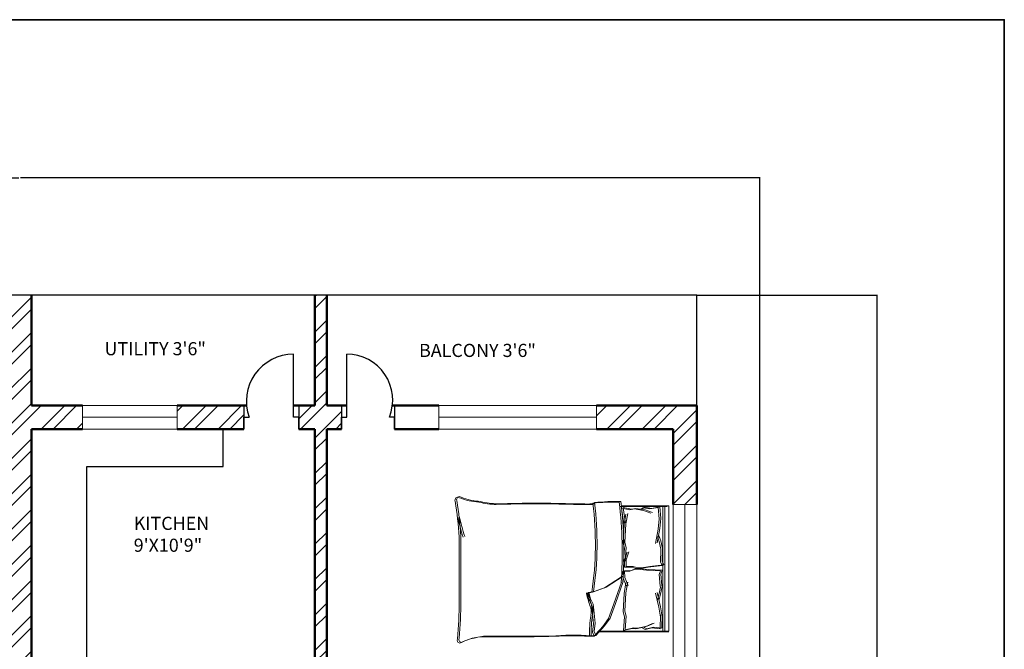
# Model space of a CAD drawing. Units: inches. Extents: x 1980 to 2738, y 1471 to 2568.
# Tile 22 of 22: x 2363 to 2738, y 2328 to 2568. Entities that reach past the tile are written whole.
import ezdxf

# ---------------------------------------------------------------- set-up
doc = ezdxf.new("R2010")
doc.units = ezdxf.units.IN
for name, color, linetype, lineweight in [('A-ANNO-DIMS', 2, 'Continuous', 18), ('A-ANNO-TTLB', 7, 'Continuous', 35), ('A-AREA-IDEN', 7, 'Continuous', 18), ('A-DOOR', 31, 'Continuous', 25), ('A-FLOR-BALC', 7, 'Continuous', 25), ('A-FLOR-CASE', 8, 'Continuous', 25), ('A-FURN', 8, 'Continuous', 18), ('A-GLAZ', 141, 'Continuous', 18), ('A-WALL', 7, 'Continuous', 50)]:
    doc.layers.add(name, color=color, linetype=linetype, lineweight=lineweight)
doc.layers.add('A-WALL-PATT', color=9, linetype='Continuous', lineweight=13, true_color=0xd19cc7)
doc.styles.get("Standard").update_dxf_attribs({"font": 'arial.ttf'})
doc.dimstyles.get("Standard").update_dxf_attribs({"dimtxt": 0.18, "dimasz": 0.18, "dimexe": 0.18, "dimexo": 0.0625, "dimgap": 0.09, "dimtad": 0, "dimtih": 1, "dimtoh": 1, "dimdec": 4, "dimzin": 0, "dimdsep": 46, "dimtxsty": 'Standard', "dimcen": 0.09, "dimadec": 0, "dimazin": 0, "dimtfac": 1, "dimtdec": 4, "dimtofl": 0, "dimtmove": 0, "dimatfit": 3, "dimfxl": 1, "dimtolj": 1, "dimtzin": 0, "dimarcsym": 0})

# ---------------------------------------------------------------- blocks, each defined once
blk = doc.blocks.new('BED-DOUBLE')
for p, q in [((27.75, 52.87), (24.5, 49.16)), ((27.75, 52.87), (24.5, 49.16)), ((28.38, 53.1), (25.13, 49.39)), ((28.38, 53.1), (25.13, 49.39)), ((29.49, 52.95), (27.75, 52.87, 3.87)), ((29.49, 52.95), (27.75, 52.87, 3.87)), ((28.36, 51.33), (27.75, 52.87)), ((28.36, 51.33), (27.75, 52.87)), ((30.13, 53.18), (28.38, 53.1, 3.87)), ((30.13, 53.18), (28.38, 53.1, 3.87)), ((29, 51.56), (28.38, 53.1)), ((29, 51.56), (28.38, 53.1)), ((0, 51.49), (0.64, 51.49)), ((0, 51.27), (26.61, 51.27)), ((0, 51.27), (26.61, 51.27)), ((0, 51.27), (0, 3.48)), ((0.64, 51.49), (27.25, 51.49)), ((0.64, 51.49), (27.25, 51.49)), ((1.53, 3.48), (1.53, 51.27)), ((1.53, 3.48), (1.53, 51.27)), ((2.17, 3.7), (2.17, 51.49)), ((2.17, 3.7), (2.17, 51.49)), ((2.56, 50.11), (2.46, 44.71)), ((2.56, 50.11), (2.46, 44.71)), ((2.56, 50.11), (5.77, 49.73)), ((2.56, 50.11), (5.77, 49.73)), ((3.2, 50.34), (3.1, 44.94)), ((3.2, 50.34), (3.1, 44.94)), ((3.2, 50.34), (6.41, 49.96)), ((3.2, 50.34), (6.41, 49.96)), ((8.26, 49.31), (5.58, 48.13)), ((8.26, 49.31), (5.58, 48.13)), ((5.77, 49.73), (8.34, 50.33)), ((5.77, 49.73), (8.34, 50.33)), ((8.9, 49.54), (6.22, 48.36)), ((8.9, 49.54), (6.22, 48.36)), ((6.41, 49.96), (8.98, 50.56)), ((6.41, 49.96), (8.98, 50.56)), ((11.83, 50.11), (8.26, 49.31)), ((11.83, 50.11), (8.26, 49.31)), ((8.34, 50.33), (9.38, 49.81)), ((8.34, 50.33), (9.38, 49.81)), ((12.47, 50.34), (8.9, 49.54)), ((12.47, 50.34), (8.9, 49.54)), ((8.98, 50.56), (10.02, 50.04)), ((8.98, 50.56), (10.02, 50.04)), ((13.43, 49.92), (11.83, 50.11)), ((13.43, 49.92), (11.83, 50.11)), ((14.07, 50.15), (12.47, 50.34)), ((14.07, 50.15), (12.47, 50.34)), ((16.57, 50.7), (13.43, 49.92)), ((16.57, 50.7), (13.43, 49.92)), ((17.21, 50.93), (14.07, 50.15)), ((17.21, 50.93), (14.07, 50.15)), ((16.17, 45.57), (16.57, 50.7)), ((16.17, 45.57), (16.57, 50.7)), ((16.81, 45.8), (17.21, 50.93)), ((16.81, 45.79), (17.21, 50.93)), ((24.5, 49.16), (22.33, 46.22)), ((24.5, 49.16), (22.33, 46.22)), ((25.13, 49.39), (22.97, 46.45)), ((25.13, 49.39), (22.97, 46.45)), ((28.06, 48.23), (28.36, 51.33)), ((28.06, 48.23), (28.36, 51.33)), ((28.69, 48.46), (29, 51.56)), ((28.69, 48.46), (29, 51.56)), ((2.46, 44.71), (2.54, 45.71)), ((2.46, 44.71), (2.54, 45.71)), ((2.54, 45.71), (3.07, 41.91)), ((2.54, 45.71), (3.07, 41.91)), ((3.1, 44.94), (3.18, 45.94)), ((3.1, 44.94), (3.18, 45.94)), ((3.18, 45.94), (3.71, 42.14)), ((3.18, 45.94), (3.71, 42.14)), ((16.73, 43.61), (16.17, 45.57)), ((16.73, 43.61), (16.17, 45.57)), ((17.37, 43.83), (16.81, 45.8)), ((17.37, 43.83), (16.81, 45.79)), ((22.33, 46.22), (20.32, 40.64)), ((22.33, 46.22), (20.32, 40.64)), ((22.97, 46.45), (20.96, 40.87)), ((22.97, 46.45), (20.96, 40.87)), ((28.36, 44.36), (28.06, 48.23)), ((28.36, 44.36), (28.06, 48.23)), ((29, 44.59), (28.69, 48.46)), ((29, 44.59), (28.69, 48.46)), ((3.07, 41.91), (4.42, 36.5)), ((3.07, 41.91), (4.42, 36.5)), ((3.71, 42.14), (5.06, 36.72)), ((3.71, 42.14), (5.06, 36.72)), ((16.29, 36.6), (16.73, 43.61)), ((16.29, 36.6), (16.73, 43.61)), ((16.93, 36.82), (17.37, 43.83)), ((16.93, 36.82), (17.37, 43.83)), ((28.83, 40.95), (28.36, 44.36)), ((28.83, 40.95), (28.36, 44.36)), ((29.47, 41.18), (29, 44.59)), ((29.47, 41.18), (29, 44.59)), ((3.67, 39.2), (3.08, 37.14)), ((3.67, 39.2), (3.08, 37.14)), ((4.31, 39.43), (3.72, 37.36)), ((4.31, 39.43), (3.72, 37.36)), ((20.32, 40.64), (17.38, 32.31)), ((20.32, 40.64), (17.38, 32.31)), ((20.96, 40.87), (18.02, 32.53)), ((20.96, 40.87), (18.02, 32.53)), ((29.76, 38.94), (28.83, 40.95)), ((29.76, 38.94), (28.83, 40.95)), ((30.4, 39.17), (29.47, 41.18)), ((30.4, 39.17), (29.47, 41.18)), ((30.38, 36.46), (29.76, 38.94)), ((30.38, 36.46), (29.76, 38.94)), ((31.02, 36.69), (30.4, 39.17)), ((31.02, 36.69), (30.4, 39.17)), ((79.24, 15.06), (79.24, 39.68)), ((79.24, 15.06), (79.24, 39.68)), ((79.88, 15.29), (79.88, 39.91)), ((79.88, 15.29), (79.88, 39.91)), ((3.08, 37.14), (2.54, 34.2)), ((3.08, 37.14), (2.54, 34.2)), ((2.54, 34.2), (2.56, 33.88)), ((2.54, 34.2), (2.56, 33.88)), ((2.56, 33.88), (2.98, 29.46)), ((2.56, 33.88), (2.98, 29.46)), ((3.72, 37.36), (3.18, 34.43)), ((3.72, 37.36), (3.18, 34.43)), ((3.18, 34.43), (3.2, 34.11)), ((3.18, 34.43), (3.2, 34.11)), ((3.2, 34.11), (3.62, 29.68)), ((3.2, 34.11), (3.62, 29.68)), ((16.74, 30.75), (15.45, 33.82)), ((16.74, 30.75), (15.45, 33.82)), ((15.63, 32.56), (16.29, 36.6)), ((15.63, 32.56), (16.29, 36.6)), ((17.38, 30.98), (16.09, 34.05)), ((17.38, 30.98), (16.09, 34.05)), ((16.27, 32.79), (16.93, 36.82)), ((16.27, 32.79), (16.93, 36.82)), ((17.38, 30.26), (23.88, 34.45)), ((17.38, 30.26), (23.88, 34.45)), ((18.02, 30.49), (24.52, 34.68)), ((18.02, 30.49), (24.52, 34.68)), ((23.88, 34.45), (28.36, 36.15)), ((23.88, 34.45), (28.36, 36.15)), ((24.52, 34.68), (29, 36.38)), ((24.52, 34.68), (29, 36.38)), ((28.36, 36.15), (30.38, 36.46)), ((28.36, 36.15), (30.38, 36.46)), ((29, 36.38), (31.02, 36.69)), ((29, 36.38), (31.02, 36.69)), ((16.89, 28.3), (16.74, 30.75)), ((16.89, 28.3), (16.74, 30.75)), ((17.53, 28.53), (17.38, 30.98)), ((17.53, 28.53), (17.38, 30.98)), ((1.87, 25.98), (7.22, 26.56)), ((1.87, 25.98), (7.22, 26.56)), ((2.98, 29.46), (2.49, 27.98)), ((2.98, 29.46), (2.49, 27.98)), ((2.49, 27.98), (7.87, 27.73)), ((2.49, 27.98), (7.87, 27.73)), ((2.51, 26.21), (7.86, 26.79)), ((2.51, 26.21), (7.86, 26.79)), ((3.62, 29.68), (3.13, 28.21)), ((3.62, 29.68), (3.13, 28.21)), ((3.13, 28.21), (8.51, 27.96)), ((3.13, 28.21), (8.51, 27.96)), ((7.22, 26.56), (10.4, 27.14)), ((7.22, 26.56), (10.4, 27.14)), ((7.86, 26.79), (11.04, 27.37)), ((7.86, 26.79), (11.04, 27.37)), ((7.87, 27.73), (11.08, 27.36)), ((7.87, 27.73), (11.08, 27.35)), ((8.51, 27.96), (11.72, 27.58)), ((8.51, 27.96), (11.72, 27.58)), ((10.4, 27.14), (11.7, 27.14)), ((10.4, 27.14), (11.7, 27.14)), ((11.04, 27.37), (12.34, 27.37)), ((11.04, 27.37), (12.34, 27.37)), ((11.08, 27.36), (12.38, 27.44)), ((11.08, 27.35), (12.38, 27.44)), ((11.7, 27.14), (13.58, 26.56)), ((11.7, 27.14), (13.58, 26.56)), ((11.72, 27.58), (13.02, 27.66)), ((11.72, 27.58), (13.02, 27.66)), ((12.34, 27.37), (14.22, 26.79)), ((12.34, 27.37), (14.22, 26.79)), ((12.38, 27.44), (14.22, 28.13)), ((12.38, 27.44), (14.22, 28.13)), ((13.02, 27.66), (14.86, 28.36)), ((13.02, 27.66), (14.86, 28.36)), ((13.58, 26.56), (16.26, 26.56)), ((13.58, 26.56), (16.26, 26.56)), ((14.22, 28.13), (16.89, 28.3)), ((14.22, 28.13), (16.89, 28.3)), ((14.22, 26.79), (16.9, 26.79)), ((14.22, 26.79), (16.9, 26.79)), ((14.86, 28.36), (17.53, 28.53)), ((14.86, 28.36), (17.53, 28.53)), ((16.26, 26.56), (16.26, 24.1)), ((16.26, 26.56), (16.26, 24.1)), ((16.9, 26.79), (16.9, 24.33)), ((16.9, 26.79), (16.9, 24.33)), ((2.45, 24.54), (1.87, 25.98)), ((2.45, 24.54), (1.87, 25.98)), ((2.3, 20.09), (2.45, 24.54)), ((2.3, 20.09), (2.45, 24.54)), ((3.09, 24.77), (2.51, 26.21)), ((3.09, 24.77), (2.51, 26.21)), ((2.94, 20.32), (3.09, 24.77)), ((2.94, 20.32), (3.09, 24.77)), ((16.26, 24.1), (15.17, 20.96)), ((16.26, 24.1), (15.17, 20.96)), ((16.9, 24.33), (15.81, 21.19)), ((16.9, 24.33), (15.81, 21.19)), ((16.17, 19.38), (16.57, 24.52)), ((16.17, 19.38), (16.57, 24.52)), ((16.81, 19.61), (17.21, 24.74)), ((16.81, 19.61), (17.21, 24.74)), ((2.3, 19.77), (2.3, 20.09)), ((2.3, 19.77), (2.3, 20.09)), ((3.03, 16.88), (2.3, 19.77)), ((3.03, 16.88), (2.3, 19.77)), ((2.94, 20), (2.94, 20.32)), ((2.94, 20), (2.94, 20.32)), ((3.67, 17.11), (2.94, 20)), ((3.67, 17.11), (2.94, 20)), ((16.73, 17.42), (16.17, 19.38)), ((16.73, 17.42), (16.17, 19.38)), ((17.37, 17.65), (16.81, 19.61)), ((17.37, 17.65), (16.81, 19.61)), ((3.75, 14.86), (3.03, 16.88)), ((3.75, 14.85), (3.03, 16.88)), ((3.32, 12.11), (4.33, 17.6)), ((3.32, 12.11), (4.33, 17.6)), ((4.39, 15.08), (3.67, 17.11)), ((4.39, 15.08), (3.67, 17.11)), ((3.96, 12.34), (4.97, 17.83)), ((3.96, 12.34), (4.97, 17.83)), ((16.29, 10.41), (16.73, 17.42)), ((16.29, 10.41), (16.73, 17.42)), ((16.93, 10.64), (17.37, 17.65)), ((16.93, 10.64), (17.37, 17.65)), ((3.03, 8.29), (3.32, 12.11)), ((3.03, 8.28), (3.32, 12.11)), ((3.67, 8.51), (3.96, 12.34)), ((3.67, 8.51), (3.96, 12.34)), ((3.01, 8.18), (3.03, 8.29)), ((3.01, 8.18), (3.03, 8.28)), ((3.34, 3.9), (3.01, 8.18)), ((3.34, 3.9), (3.01, 8.18)), ((3.65, 8.41), (3.67, 8.51)), ((3.65, 8.41), (3.67, 8.51)), ((3.98, 4.13), (3.65, 8.41)), ((3.98, 4.13), (3.65, 8.41)), ((15.63, 6.38), (16.29, 10.41)), ((15.63, 6.38), (16.29, 10.41)), ((16.27, 6.61), (16.93, 10.64)), ((16.27, 6.61), (16.93, 10.64)), ((16.29, 10.41), (16.62, 9.28)), ((16.29, 10.41), (16.62, 9.28)), ((16.62, 9.28), (17.34, 4.18)), ((16.62, 9.28), (17.34, 4.18)), ((16.93, 10.64), (17.26, 9.51)), ((16.93, 10.64), (17.26, 9.51)), ((17.26, 9.51), (17.98, 4.41)), ((17.26, 9.51), (17.98, 4.41)), ((3.32, 3.89), (6.5, 4.47)), ((3.32, 3.89), (6.5, 4.47)), ((3.96, 4.12), (7.14, 4.7)), ((3.96, 4.12), (7.14, 4.7)), ((8.95, 5.05), (6.21, 6.06)), ((8.95, 5.05), (6.21, 6.06)), ((6.5, 4.47), (9.1, 4.04)), ((6.5, 4.47), (9.1, 4.04)), ((9.59, 5.28), (6.85, 6.29)), ((9.59, 5.28), (6.85, 6.29)), ((7.14, 4.7), (9.74, 4.27)), ((7.14, 4.7), (9.74, 4.27)), ((12.57, 4.47), (8.95, 5.05)), ((12.57, 4.47), (8.95, 5.05)), ((9.1, 4.04), (10.11, 4.62)), ((9.1, 4.04), (10.11, 4.62)), ((13.21, 4.7), (9.59, 5.28)), ((13.21, 4.7), (9.59, 5.28)), ((9.74, 4.27), (10.75, 4.85)), ((9.74, 4.27), (10.75, 4.85)), ((14.16, 4.76), (12.57, 4.47)), ((14.16, 4.76), (12.57, 4.47)), ((14.8, 4.99), (13.21, 4.7)), ((14.8, 4.99), (13.21, 4.7)), ((17.34, 4.18), (14.16, 4.76)), ((17.34, 4.18), (14.16, 4.76)), ((17.98, 4.41), (14.8, 4.99)), ((17.98, 4.41), (14.8, 4.99)), ((18.11, 3.48), (0, 3.48)), ((18.11, 3.48), (0, 3.48)), ((18.75, 3.7), (0.64, 3.7)), ((18.75, 3.7), (0.64, 3.7))]:
    blk.add_line(p, q)
for centre, radius, start, end in [((-6.66, 51.33), 36.18, 349.8763, 2.5657), ((-6.66, 51.33), 36.18, 349.8763, 2.5657), ((36.31, 182.27), 129.5, 266.9791, 273.8365), ((36.31, 182.27), 129.5, 266.9791, 273.8365), ((-6.02, 51.56), 36.18, 349.8763, 2.5657), ((-6.02, 51.56), 36.18, 349.8763, 2.5657), ((36.95, 182.49), 129.5, 266.9791, 273.8365), ((36.95, 182.49), 129.5, 266.9791, 273.8365), ((67.82, -4508.74), 4561.86, 90.00217, 90.28689), ((67.82, -4508.74), 4561.86, 90.00217, 90.28689), ((68.46, -4508.51), 4561.86, 90.00217, 90.28689), ((68.46, -4508.52), 4561.86, 90.00217, 90.28689), ((68.67, 76.16), 23.07, 267.4714, 296.4681), ((68.67, 76.16), 23.07, 267.4714, 296.4681), ((69.31, 76.39), 23.07, 267.4714, 296.4681), ((69.31, 76.39), 23.07, 267.4714, 296.4681), ((78.87, 54.41), 1.1, 332.6588, 86.02), ((78.87, 54.41), 1.1, 332.6588, 86.02), ((212.28, 41.15), 133.04, 174.4998, 180.6351), ((212.28, 41.15), 133.04, 174.4998, 180.6351), ((79.51, 54.64), 1.1, 332.6588, 86.02), ((79.51, 54.64), 1.1, 332.6588, 86.02), ((212.92, 41.38), 133.04, 174.4998, 180.6351), ((212.92, 41.38), 133.04, 174.4998, 180.6351), ((35.71, 43.97), 6.22, 168.6608, 203.7384), ((35.71, 43.97), 6.22, 168.6608, 203.7384), ((35.07, 43.74), 6.22, 168.6608, 203.7384), ((35.07, 43.74), 6.22, 168.6608, 203.7384), ((2.12, 31.38), 29.65, 10.6617, 19.8806), ((2.12, 31.38), 29.65, 10.6617, 19.8806), ((1.48, 31.15), 29.65, 10.6617, 19.8806), ((1.48, 31.15), 29.65, 10.6617, 19.8806), ((156.32, 17.76), 129.02, 171.7845, 186.9006), ((156.32, 17.76), 129.02, 171.7845, 186.9006), ((156.96, 17.98), 129.02, 171.7845, 186.9006), ((156.96, 17.98), 129.02, 171.7845, 186.9006), ((30.44, 36.64), 0.185, 250.2464, 1.1377), ((30.44, 36.64), 0.185, 250.2464, 1.1377), ((31.08, 36.86), 0.185, 250.2464, 1.1377), ((31.08, 36.86), 0.185, 250.2464, 1.1377), ((182.05, 21.36), 164.97, 176.0865, 186.7821), ((182.05, 21.36), 164.97, 176.0865, 186.7821), ((182.69, 21.59), 164.97, 176.0865, 186.7821), ((182.69, 21.59), 164.97, 176.0865, 186.7821), ((-23.71, -17.22), 106.46, 13.3832, 17.7053), ((-23.71, -17.22), 106.46, 13.3832, 17.7053), ((-23.07, -16.99), 106.46, 13.3832, 17.7053), ((-23.07, -16.99), 106.46, 13.3832, 17.7053), ((200.84, 21.43), 121.76, 182.9958, 189.4091), ((200.84, 21.43), 121.76, 182.9958, 189.4091), ((201.48, 21.66), 121.76, 182.9958, 189.4091), ((201.48, 21.66), 121.76, 182.9958, 189.4091), ((20.1, 85.16), 83.31, 268.7218, 275.604), ((20.1, 85.16), 83.31, 268.7218, 275.604), ((20.74, 85.39), 83.31, 268.7218, 275.604), ((20.74, 85.39), 83.31, 268.7218, 275.604), ((31.17, -167.31), 170.11, 88.4762, 91.0082), ((31.17, -167.31), 170.11, 88.4762, 91.0082), ((31.81, -167.08), 170.11, 88.4762, 91.0082), ((31.81, -167.08), 170.11, 88.4762, 91.0082), ((50.61, 484.82), 482.31, 268.2277, 271.7185), ((50.61, 484.82), 482.31, 268.2277, 271.7185), ((51.25, 485.05), 482.31, 268.2277, 271.7185), ((51.25, 485.05), 482.31, 268.2277, 271.7185), ((64.51, -26.9), 29.63, 76.0648, 88.9113), ((64.51, -26.9), 29.63, 76.0648, 88.9113), ((65.15, -26.67), 29.63, 76.0648, 88.9113), ((65.15, -26.67), 29.63, 76.0648, 88.9113), ((70.28, -21.66), 23.56, 67.9751, 86.652), ((70.28, -21.66), 23.56, 67.9751, 86.652), ((70.91, -21.43), 23.56, 67.9751, 86.652), ((70.91, -21.43), 23.56, 67.9751, 86.652), ((79.72, 1.09), 1.09, 236.1736, 23.4781), ((79.72, 1.09), 1.09, 236.1736, 23.4781), ((80.36, 1.32), 1.09, 236.1736, 23.4781), ((80.36, 1.32), 1.09, 236.1736, 23.4781)]:
    blk.add_arc(centre, radius, start, end)
blk = doc.blocks.new('WIN-60IN-WALL')
for p, q in [((0, 9), (0, 0)), ((60, 9), (0, 9)), ((60, 4.5), (60, 9)), ((60, 9), (60, 0)), ((0, 0), (0, 4.5)), ((0, 4.5), (60, 4.5)), ((0, 0), (60, 0))]:
    blk.add_line(p, q)
blk = doc.blocks.new('WIN-36IN-WALL')
for p, q in [((0, 9), (0, 0)), ((0, 9), (36, 9)), ((36, 4.5), (36, 9)), ((36, 9), (36, 0)), ((0, 0), (0, 4.5)), ((0, 4.5), (36, 4.5)), ((36, 0), (0, 0))]:
    blk.add_line(p, q)
blk = doc.blocks.new('*D35')
at = {"layer": 'A-ANNO-DIMS', "color": 0, "lineweight": -2, "transparency": 16777216}
for p, q in [((2081.08, 2291.77), (2081.08, 2507.54)), ((2081.26, 2507.36), (2362.79, 2507.36)), ((2644.9, 2507.36), (2363.37, 2507.36)), ((2645.08, 2291.77), (2645.08, 2507.54))]:
    blk.add_line(p, q, dxfattribs=at)
at = {"layer": 'A-ANNO-DIMS', "color": 0, "transparency": 16777216}
for points in [[(2081.26, 2507.39), (2081.26, 2507.33), (2081.08, 2507.36)], [(2644.9, 2507.39), (2644.9, 2507.33), (2645.08, 2507.36)]]:
    blk.add_solid(points, dxfattribs=at)
at = {"layer": 'Defpoints', "color": 0, "transparency": 16777216}
for p in [(2645.08, 2507.36), (2081.08, 2291.71), (2645.08, 2291.71)]:
    blk.add_point(p, dxfattribs=at)
at = {"layer": 'A-ANNO-DIMS', "color": 0, "transparency": 16777216, "insert": (2363.08, 2507.36), "char_height": 0.18, "attachment_point": 5}
blk.add_mtext('\\A1;564', dxfattribs=at)
blk = doc.blocks.new('*D39')
at = {"layer": 'A-ANNO-DIMS', "color": 0, "lineweight": -2, "transparency": 16777216}
for p, q in [((2621.15, 2462.71), (2689.91, 2462.71)), ((2689.73, 2462.53), (2689.73, 2279.14)), ((2689.73, 2095.39), (2689.73, 2278.77)), ((2579.97, 2095.21), (2689.91, 2095.21))]:
    blk.add_line(p, q, dxfattribs=at)
at = {"layer": 'A-ANNO-DIMS', "color": 0, "transparency": 16777216}
for points in [[(2689.7, 2462.53), (2689.76, 2462.53), (2689.73, 2462.71)], [(2689.7, 2095.39), (2689.76, 2095.39), (2689.73, 2095.21)]]:
    blk.add_solid(points, dxfattribs=at)
at = {"layer": 'Defpoints', "color": 0, "transparency": 16777216}
for p in [(2621.08, 2462.71), (2689.73, 2462.71), (2579.9, 2095.21)]:
    blk.add_point(p, dxfattribs=at)
at = {"layer": 'A-ANNO-DIMS', "color": 0, "transparency": 16777216, "insert": (2689.73, 2278.96), "char_height": 0.18, "attachment_point": 5}
blk.add_mtext('\\A1;367.5', dxfattribs=at)

msp = doc.modelspace()

# ---------------------------------------------------------------- hatches: boundary and pattern name
at = {"layer": 'A-WALL-PATT'}
h = msp.add_hatch(dxfattribs=at)
h.set_pattern_fill('ANSI32', color=256)
h.paths.add_polyline_path([(2257.5661, 2416.2064), (2257.5661, 2420.7064), (2250.5833, 2420.7064), (2250.5833, 2462.7064), (2246.0833, 2462.7064), (2246.0833, 2420.7064), (2237.0791, 2420.7064), (2237.0791, 2411.7064), (2246.0833, 2411.7064), (2246.0833, 2291.7064), (2242.6109, 2291.7064), (2242.6109, 2287.2064), (2246.0833, 2287.2064), (2250.5833, 2287.2064), (2250.5833, 2291.7064), (2250.5833, 2411.7064), (2257.5661, 2411.7064)])
h.paths.add_polyline_path([(2387.0396, 2416.2064), (2387.0396, 2420.7064), (2367.5833, 2420.7064), (2367.5833, 2462.7064), (2358.5833, 2462.7064), (2358.5833, 2420.7064), (2329.3087, 2420.7064), (2329.3087, 2411.7064), (2358.5833, 2411.7064), (2358.5833, 2321.7275), (2358.5833, 2309.7064), (2347.3089, 2309.7064), (2293.3089, 2309.7064), (2293.3089, 2259.0771), (2297.8089, 2259.0771), (2297.8089, 2305.2064), (2347.3089, 2305.2064), (2347.3089, 2284.7412), (2351.8089, 2284.7412), (2351.8089, 2305.2064), (2372.3188, 2305.2064), (2372.3761, 2284.3899), (2377.0295, 2284.3899), (2377.0295, 2299.3058), (2377.0295, 2305.2064), (2426.5295, 2305.2064), (2426.5295, 2257.5573), (2431.0295, 2257.5573), (2431.0295, 2309.7064), (2377.0295, 2309.7064), (2367.5833, 2309.7064), (2367.5833, 2321.7275), (2367.5833, 2411.7064), (2387.0396, 2411.7064)])
h.paths.add_polyline_path([(2448.5267, 2416.2064), (2448.5267, 2420.7064), (2423.0396, 2420.7064), (2423.0396, 2411.7064), (2448.5267, 2411.7064)])
h.paths.add_polyline_path([(2130.9128, 2416.2064), (2130.9128, 2420.7064), (2105.0833, 2420.7064), (2105.0833, 2386.6942), (2114.0833, 2386.6942), (2114.0833, 2411.7064), (2130.9128, 2411.7064)])
h.paths.add_polyline_path([(2212.9478, 2420.7064), (2190.9128, 2420.7064), (2190.9128, 2411.7064), (2212.9478, 2411.7064), (2212.9478, 2416.2064)])
h.paths.add_polyline_path([(2114.0833, 2326.6942), (2105.0833, 2326.6942), (2105.0833, 2291.7064), (2081.0833, 2291.7064), (2081.0833, 2287.2064), (2105.0833, 2287.2064), (2105.0833, 2276.1935), (2114.0833, 2276.1935), (2114.0833, 2287.2064), (2166.3825, 2287.2064), (2166.3825, 2289.4564), (2166.3825, 2291.7064), (2114.0833, 2291.7064)])
h.paths.add_polyline_path([(2114.0833, 2252.1935), (2105.0833, 2252.1935), (2105.0833, 2233.2064), (2081.0833, 2233.2064), (2081.0833, 2228.7064), (2105.0833, 2228.7064), (2105.0833, 2213.4478), (2114.0833, 2213.4478), (2114.0833, 2228.7064), (2195.0833, 2228.7064), (2199.5833, 2228.7064), (2208.4455, 2228.7064), (2208.4455, 2230.9564), (2208.4455, 2233.2064), (2199.5833, 2233.2064), (2199.5833, 2287.2064), (2206.8904, 2287.2064), (2206.8904, 2289.4564), (2206.8904, 2291.7064), (2189.446, 2291.7064), (2189.446, 2289.4564), (2189.446, 2287.2064), (2195.0833, 2287.2064), (2195.0833, 2233.2064), (2114.0833, 2233.2064)])
h.paths.add_polyline_path([(2114.0833, 2153.4478), (2109.5833, 2153.4478), (2105.0833, 2153.4478), (2105.0833, 2135.2374), (2114.0833, 2135.2374)], flags=17)
h.paths.add_polyline_path([(2135.9619, 2095.4081), (2140.1805, 2095.4081), (2140.1805, 2104.2064), (2114.0833, 2104.2064), (2114.0833, 2110.3997), (2109.5833, 2110.3997), (2105.0833, 2110.3997), (2105.0833, 2104.2064), (2081.0833, 2104.2064), (2081.0833, 2099.7064), (2105.0833, 2099.7064), (2127.5416, 2099.8532), (2127.5416, 2056.9393), (2136.2133, 2056.9393)], flags=17)
h.paths.add_polyline_path([(2255.4895, 2104.2064), (2250.5833, 2104.2064), (2250.5833, 2233.2064), (2246.0833, 2233.2064), (2242.4941, 2233.2064), (2242.4941, 2228.7064), (2246.0833, 2228.7064), (2246.0833, 2104.2064), (2163.6825, 2104.2064), (2163.6825, 2099.8072), (2163.6825, 2095.4081), (2191.4325, 2095.4081), (2191.4325, 2011.2064), (2186.0833, 2011.2064), (2136.5143, 2010.8824), (2136.3702, 2032.9403), (2131.9559, 2032.9115), (2127.5416, 2032.8826), (2127.5416, 2006.7064), (2105.0833, 2006.7064), (2081.0833, 2006.7064), (2081.0833, 2002.2064), (2105.0833, 2002.2064), (2105.0833, 1995.9329), (2114.0833, 1995.9329), (2114.0833, 2002.2064), (2246.0833, 2002.2064), (2246.0833, 1877.7064), (2242.1358, 1877.7064), (2242.1358, 1873.2064), (2250.5833, 1873.2064), (2250.5833, 2002.2064), (2255.3335, 2002.2064), (2255.3335, 2011.2064), (2195.9325, 2011.2064), (2195.9325, 2095.2064), (2255.4895, 2095.2064), (2255.4895, 2099.5471)])
h.paths.add_polyline_path([(2199.5833, 1873.2064), (2209.827, 1873.2064), (2209.827, 1875.4564), (2209.827, 1877.7064), (2114.0833, 1877.7064), (2114.0833, 1890.0968), (2105.0833, 1890.0968), (2105.0833, 1877.7064), (2081.0833, 1877.7064), (2081.0833, 1873.2064), (2105.0833, 1873.2064), (2105.0833, 1857.7279), (2114.0833, 1857.7279), (2114.0833, 1873.2064), (2195.0833, 1873.2064), (2195.0833, 1819.2064), (2190.298, 1819.2064), (2190.298, 1814.7064), (2209.8976, 1814.7064), (2209.8976, 1816.9564), (2209.8976, 1819.2064), (2199.5833, 1819.2064)])
h.paths.add_polyline_path([(2114.0833, 1814.7064), (2166.2538, 1814.7064), (2166.2538, 1816.9564), (2166.2538, 1819.2064), (2114.0833, 1819.2064), (2114.0833, 1833.7279), (2109.5833, 1833.7279), (2105.0833, 1833.7279), (2105.0833, 1819.2064), (2081.0833, 1819.2064), (2081.0833, 1814.7064), (2105.0833, 1814.7064), (2105.0833, 1782.5516), (2114.0833, 1782.5516)])
h.paths.add_polyline_path([(2114.0833, 1722.5516), (2109.5833, 1722.5516), (2105.0833, 1722.5516), (2105.0833, 1685.7064), (2124.5104, 1685.7064), (2124.5104, 1690.2064), (2124.5104, 1694.7064), (2114.0833, 1694.7064)])
h.paths.add_polyline_path([(2218.8787, 1694.7064), (2184.5104, 1694.7064), (2184.5104, 1685.7064), (2218.8787, 1685.7064), (2218.8787, 1690.2064)])
h.paths.add_polyline_path([(2250.5833, 1819.2064), (2242.6431, 1819.2064), (2242.6431, 1816.9564), (2242.6431, 1814.7064), (2246.0833, 1814.7064), (2246.0833, 1694.7064), (2240.4035, 1694.7064), (2240.4035, 1690.2064), (2240.4035, 1685.7064), (2246.0833, 1685.7064), (2246.0833, 1643.7064), (2250.5833, 1643.7064), (2250.5833, 1685.7064), (2255.9859, 1685.7064), (2255.9859, 1690.2064), (2255.9859, 1694.7064), (2250.5833, 1694.7064)])
h.paths.add_polyline_path([(2297.4764, 1694.7064), (2279.3934, 1694.7064), (2279.3934, 1690.2064), (2279.3934, 1685.7064), (2297.4764, 1685.7064), (2297.4764, 1690.2064)])
h.paths.add_polyline_path([(2377.1596, 1694.7064), (2367.5833, 1694.7064), (2367.5833, 1787.7064), (2431.0295, 1787.7064), (2431.0295, 1792.2064), (2431.0295, 1849.4149), (2428.7795, 1849.4149), (2426.5295, 1849.4149), (2426.5295, 1792.2064), (2421.5833, 1792.2064), (2367.5833, 1792.2064), (2297.8089, 1792.2064), (2297.8089, 1850.2946), (2295.5589, 1850.2946), (2293.3089, 1850.2946), (2293.3089, 1792.2064), (2293.3089, 1787.7064), (2297.8089, 1787.7064), (2358.5833, 1787.7064), (2358.5833, 1694.7064), (2333.4764, 1694.7064), (2333.4764, 1685.7064), (2358.5833, 1685.7064), (2358.5833, 1643.7064), (2367.5833, 1643.7064), (2367.5833, 1685.7064), (2377.1596, 1685.7064)])
h.paths.add_polyline_path([(2442.4912, 1694.7064), (2413.1596, 1694.7064), (2413.1596, 1685.7064), (2442.4912, 1685.7064)])
h.paths.add_polyline_path([(2480.0833, 1814.7064), (2483.4816, 1814.7064), (2483.4816, 1817.9384), (2483.4816, 1819.2064), (2475.5833, 1819.2064), (2475.5833, 1694.7064), (2470.7283, 1694.7064), (2470.7283, 1685.7064), (2475.5833, 1685.7064), (2475.5833, 1643.7064), (2480.0833, 1643.7064), (2480.0833, 1685.7064), (2486.3293, 1685.7064), (2486.3293, 1690.2064), (2486.3293, 1694.7064), (2480.0833, 1694.7064)])
h.paths.add_polyline_path([(2621.0833, 1721.7349), (2612.0833, 1721.7349), (2612.0833, 1694.7064), (2586.1453, 1694.7064), (2586.1453, 1685.7064), (2621.0833, 1685.7064)])
h.paths.add_polyline_path([(2526.1453, 1690.2064), (2526.1453, 1694.7064), (2511.584, 1694.7064), (2511.584, 1690.2064), (2511.584, 1685.7064), (2526.1453, 1685.7064)])
h.paths.add_polyline_path([(2645.0833, 1819.2064), (2621.0833, 1819.2064), (2621.0833, 1835.8527), (2616.5833, 1835.8527), (2612.0833, 1835.8527), (2612.0833, 1819.2064), (2560.2541, 1819.2064), (2560.2541, 1814.7064), (2612.0833, 1814.7064), (2612.0833, 1781.7349), (2621.0833, 1781.7349), (2621.0833, 1814.7064), (2645.0833, 1814.7064)])
h.paths.add_polyline_path([(2645.0833, 1877.7064), (2621.0833, 1877.7064), (2621.0833, 1886.4375), (2612.0833, 1886.4375), (2612.0833, 1877.7064), (2517.1032, 1877.7064), (2517.1032, 1875.4564), (2517.1032, 1873.2064), (2526.5833, 1873.2064), (2526.5833, 1819.2064), (2516.6454, 1819.2064), (2516.6454, 1816.9564), (2516.6454, 1814.7064), (2536.4445, 1814.7064), (2536.4445, 1816.9564), (2536.4445, 1819.2064), (2531.0833, 1819.2064), (2531.0833, 1873.2064), (2612.0833, 1873.2064), (2612.0833, 1859.8527), (2621.0833, 1859.8527), (2621.0833, 1873.2064), (2645.0833, 1873.2064)])
h.paths.add_polyline_path([(2645.0833, 2006.7064), (2621.0833, 2006.7064), (2588.5085, 2006.7064), (2588.5085, 2052.9125), (2579.9045, 2052.9125), (2579.9045, 2011.2064), (2519.9045, 2011.2064), (2519.9045, 2095.2064), (2553.1204, 2095.2064), (2553.1204, 2104.2064), (2480.0833, 2104.2064), (2480.0833, 2228.7064), (2484.3832, 2228.7064), (2484.3832, 2230.9564), (2484.3832, 2233.2064), (2475.5833, 2233.2064), (2475.5833, 2104.2064), (2463.1308, 2104.2064), (2463.1308, 2095.2064), (2501.2463, 2095.2064), (2510.9045, 2095.2064), (2515.4045, 2095.2064), (2515.4045, 2011.2064), (2510.9045, 2011.2064), (2501.2463, 2011.2064), (2462.5957, 2011.2064), (2462.5957, 2002.2064), (2475.5833, 2002.2064), (2475.5833, 1873.2064), (2483.6146, 1873.2064), (2483.6146, 1875.4564), (2483.6146, 1877.7064), (2480.0833, 1877.7064), (2480.0833, 2002.2064), (2612.0833, 2002.2064), (2612.0833, 1996.309), (2621.0833, 1996.309), (2621.0833, 2002.2064), (2645.0833, 2002.2064)])
h.paths.add_polyline_path([(2588.5085, 2099.7277), (2621.0833, 2099.7277), (2645.0833, 2099.7064), (2645.0833, 2104.2064), (2621.0833, 2104.2064), (2621.0833, 2109.0038), (2616.5833, 2109.0038), (2612.0833, 2109.0038), (2612.0833, 2104.2064), (2575.0621, 2104.2064), (2575.0621, 2099.7064), (2575.0621, 2095.2064), (2579.9045, 2095.2064), (2579.9045, 2076.9125), (2588.5085, 2076.9125)], flags=17)
h.paths.add_polyline_path([(2367.5833, 2002.2064), (2373.7228, 2002.2064), (2373.7228, 2006.7064), (2373.7228, 2011.2064), (2350.7889, 2011.2064), (2350.7889, 2006.7064), (2350.7889, 2002.2064), (2358.5833, 2002.2064), (2358.5833, 1877.7064), (2293.3089, 1877.7064), (2293.3089, 1870.4987), (2297.8089, 1870.4987), (2297.8089, 1873.2064), (2347.3089, 1873.2064), (2347.3089, 1847.2208), (2351.8089, 1847.2208), (2351.8089, 1873.2064), (2372.5295, 1873.2064), (2372.5295, 1847.8619), (2377.0295, 1847.8619), (2377.0295, 1873.2064), (2426.5295, 1873.2064), (2426.5295, 1868.7339), (2431.0295, 1868.7339), (2431.0295, 1877.7064), (2367.5833, 1877.7064)])
h.paths.add_polyline_path([(2531.0833, 2287.2064), (2534.2285, 2287.2064), (2534.2285, 2291.7064), (2516.7886, 2291.7064), (2516.7886, 2287.2064), (2526.5833, 2287.2064), (2526.5833, 2233.2064), (2517.9112, 2233.2064), (2517.9112, 2230.9564), (2517.9112, 2228.7064), (2526.5833, 2228.7064), (2531.0833, 2228.7064), (2612.0833, 2228.7064), (2612.0833, 2206.8504), (2621.0833, 2206.8504), (2621.0833, 2228.7064), (2645.0833, 2228.7064), (2645.0833, 2233.2064), (2621.0833, 2233.2064), (2621.0833, 2241.8536), (2616.5833, 2241.8536), (2612.0833, 2241.8536), (2612.0833, 2233.2064), (2531.0833, 2233.2064)])
h.paths.add_polyline_path([(2645.0833, 2291.7064), (2621.0833, 2291.7064), (2621.0833, 2323.0138), (2616.5833, 2323.0138), (2612.0833, 2323.0138), (2612.0833, 2291.7064), (2559.6852, 2291.7064), (2559.6852, 2289.4564), (2559.6852, 2287.2064), (2612.0833, 2287.2064), (2612.0833, 2265.8536), (2621.0833, 2265.8536), (2621.0833, 2287.2064), (2645.0833, 2287.2064)])
h.paths.add_polyline_path([(2621.0833, 2420.7064), (2582.8189, 2420.7064), (2582.8189, 2411.7064), (2612.0833, 2411.7064), (2612.0833, 2383.0138), (2621.0833, 2383.0138)])
h.paths.add_polyline_path([(2480.0833, 2411.7064), (2485.7342, 2411.7064), (2485.7342, 2416.2064), (2485.7342, 2420.7064), (2480.0833, 2420.7064), (2480.0833, 2462.7064), (2475.5833, 2462.7064), (2475.5833, 2420.7064), (2469.4083, 2420.7064), (2469.4083, 2411.7064), (2475.5833, 2411.7064), (2475.5833, 2291.7064), (2475.5833, 2287.2064), (2482.9195, 2287.2064), (2482.9195, 2289.4564), (2482.9195, 2291.7064), (2480.0833, 2291.7064)])
h.paths.add_polyline_path([(2367.5833, 2228.7064), (2431.0295, 2228.7064), (2431.0295, 2233.2064), (2431.0295, 2237.4203), (2428.7795, 2237.4203), (2426.5295, 2237.4203), (2426.5295, 2233.2064), (2377.0295, 2233.2064), (2377.0295, 2260.3837), (2372.4423, 2260.3837), (2372.517, 2233.2635), (2351.8089, 2233.2064), (2351.8089, 2260.7412), (2347.3089, 2260.7412), (2347.3089, 2233.2064), (2297.8089, 2233.2064), (2297.8089, 2236.9324), (2293.3089, 2236.9324), (2293.3089, 2228.7064), (2358.5833, 2228.7064), (2358.5833, 2104.2064), (2353.3665, 2104.2064), (2353.3665, 2095.2064), (2373.8869, 2095.2064), (2373.8869, 2099.7064), (2373.8869, 2104.2064), (2367.5833, 2104.2064)])
h.paths.add_polyline_path([(2321.2323, 2104.2064), (2303.4895, 2104.2064), (2303.4895, 2095.2064), (2321.2323, 2095.2064), (2321.2323, 2099.7064)], flags=0)
h.paths.add_polyline_path([(2415.1308, 2099.7064), (2415.1308, 2104.2064), (2404.81, 2104.2064), (2404.81, 2095.2064), (2415.1308, 2095.2064)], flags=17)
h.paths.add_polyline_path([(2318.6336, 2011.2064), (2303.3335, 2011.2064), (2303.3335, 2002.2064), (2318.6336, 2002.2064)], flags=0)
h.paths.add_polyline_path([(2414.5957, 2011.2064), (2406.2461, 2011.2064), (2406.2461, 2006.7064), (2406.2461, 2002.2064), (2414.5957, 2002.2064)], flags=17)

# ---------------------------------------------------------------- linework, layer by layer
at = {"layer": 'A-ANNO-TTLB'}
msp.add_lwpolyline([(1979.5621, 2567.5568), (2738.2543, 2567.5568), (2738.2543, 1471.317), (1979.5621, 1471.317)], close=True, dxfattribs=at)
at = {"layer": 'A-DOOR'}
for p, q in [((2467.4083, 2416.2064), (2467.4083, 2440.2064)), ((2487.7342, 2416.2064), (2487.7342, 2440.2064)), ((2448.5267, 2420.7064), (2448.5267, 2411.7064)), ((2469.4083, 2420.7064), (2469.4083, 2411.7064)), ((2485.7342, 2420.7064), (2485.7342, 2411.7064)), ((2505.9478, 2420.7064), (2505.9478, 2411.7064)), ((2448.5267, 2411.7064), (2448.5267, 2416.2064)), ((2448.5267, 2416.2064), (2450.5267, 2416.2064)), ((2469.4083, 2416.2064), (2467.4083, 2416.2064)), ((2469.4083, 2411.7064), (2469.4083, 2416.2064)), ((2485.7342, 2411.7064), (2485.7342, 2416.2064)), ((2485.7342, 2416.2064), (2487.7342, 2416.2064)), ((2505.9478, 2416.2064), (2503.9478, 2416.2064)), ((2505.9478, 2411.7064), (2505.9478, 2416.2064))]:
    msp.add_line(p, q, dxfattribs=at)
for centre, radius, start, end in [((2467.4083, 2422.2692), 17.9373, 90, 199.754859), ((2487.7342, 2422.7298), 17.4767, 338.083178, 90)]:
    msp.add_arc(centre, radius, start, end, dxfattribs=at)
at = {"layer": 'A-FLOR-BALC'}
for p, q in [((2621.0833, 2462.7064), (2250.5833, 2462.7064)), ((2621.0833, 2420.7064), (2621.0833, 2462.7064))]:
    msp.add_line(p, q, dxfattribs=at)
at = {"layer": 'A-FLOR-CASE'}
for p, q in [((2440.5957, 2397.4159), (2440.5957, 2411.7064)), ((2388.6126, 2309.7064), (2388.6126, 2397.4159)), ((2388.6126, 2397.4159), (2440.5957, 2397.4159))]:
    msp.add_line(p, q, dxfattribs=at)
at = {"layer": 'A-WALL'}
for p, q in [((2367.5833, 2420.7064), (2367.5833, 2462.7064)), ((2475.5833, 2420.7064), (2475.5833, 2462.7064)), ((2475.5833, 2462.7064), (2475.5833, 2462.7064)), ((2480.0833, 2420.7064), (2480.0833, 2462.7064)), ((2367.5833, 2420.7064), (2387.0396, 2420.7064)), ((2367.5833, 2420.7064), (2387.0396, 2420.7064)), ((2423.0396, 2420.7064), (2449.5392, 2420.7064)), ((2423.0396, 2420.7064), (2449.5392, 2420.7064)), ((2467.4083, 2420.7064), (2475.5833, 2420.7064)), ((2467.4083, 2420.7064), (2475.5833, 2420.7064)), ((2480.0833, 2420.7064), (2487.7342, 2420.7064)), ((2480.0833, 2420.7064), (2487.7342, 2420.7064)), ((2505.0934, 2420.7064), (2522.8189, 2420.7064)), ((2505.0934, 2420.7064), (2522.8189, 2420.7064)), ((2582.8189, 2420.7064), (2621.0833, 2420.7064)), ((2582.8189, 2420.7064), (2621.0833, 2420.7064)), ((2621.0833, 2420.7064), (2621.0833, 2383.0138)), ((2367.5833, 2411.7064), (2367.5833, 2321.7275)), ((2367.5833, 2411.7064), (2387.0396, 2411.7064)), ((2423.0396, 2411.7064), (2448.5267, 2411.7064)), ((2469.4083, 2411.7064), (2475.5833, 2411.7064)), ((2475.5833, 2411.7064), (2475.5833, 2291.7064)), ((2475.5833, 2411.7064), (2475.5833, 2411.7064)), ((2480.0833, 2411.7064), (2480.0833, 2291.7064)), ((2480.0833, 2411.7064), (2485.7342, 2411.7064)), ((2505.9478, 2411.7064), (2522.8189, 2411.7064)), ((2582.8189, 2411.7064), (2612.0833, 2411.7064)), ((2612.0833, 2411.7064), (2612.0833, 2383.0138))]:
    msp.add_line(p, q, dxfattribs=at)

# ---------------------------------------------------------------- block references
at = {"layer": 'A-FURN', "rotation": 180}
msp.add_blockref('BED-DOUBLE', (2610.3724, 2385.9598), dxfattribs=at)
at = {"layer": 'A-GLAZ'}
msp.add_blockref('WIN-36IN-WALL', (2387.04, 2411.706), dxfattribs=at)
for p, rotation in [((2582.8187, 2420.7068), 180), ((2612.0828, 2383.0136), 270)]:
    msp.add_blockref('WIN-60IN-WALL', p, dxfattribs=dict(at, rotation=rotation))

# ---------------------------------------------------------------- texts
at = {"layer": 'A-AREA-IDEN', "char_height": 5, "attachment_point": 1}
for s, width, insert in [('UTILITY 3\'6"', 173.533722, (2395.3923, 2444.7943)), ('BALCONY 3\'6"', 160.508814, (2515.2477, 2444.1368)), ('KITCHEN\\P9\'X10\'9"', 73.550432, (2406.5328, 2378.2959))]:
    msp.add_mtext_dynamic_manual_height_columns(s, width=width, gutter_width=12.5, heights=[0], dxfattribs=dict(at, insert=insert))

# ---------------------------------------------------------------- dimensions: what is measured, and where the dimension line sits
at = {"layer": 'A-ANNO-DIMS'}
dim = msp.add_linear_dim(base=(2645.0833, 2507.3564), p1=(2081.0833, 2291.7064), p2=(2645.0833, 2291.7064), dimstyle='Standard', override={"dimdec": 0, "dimlfac": 1, "dimrnd": 0, "dimzin": 0, "dimdsep": 46, "dimlunit": 2}, dxfattribs=at)
dim.commit()
dim.dimension.update_dxf_attribs({"geometry": '*D35', "text_midpoint": (2363.0833, 2507.3564)})
dim = msp.add_linear_dim(base=(2689.7333, 2462.7064), p1=(2579.9045, 2095.2064), p2=(2621.0833, 2462.7064), angle=90, dimstyle='Standard', override={"dimdec": 1, "dimlfac": 1, "dimrnd": 0, "dimzin": 0, "dimdsep": 46, "dimlunit": 2}, dxfattribs=at)
dim.commit()
dim.dimension.update_dxf_attribs({"geometry": '*D39', "text_midpoint": (2689.7333, 2278.9564)})

doc.saveas('drawing.dxf')
